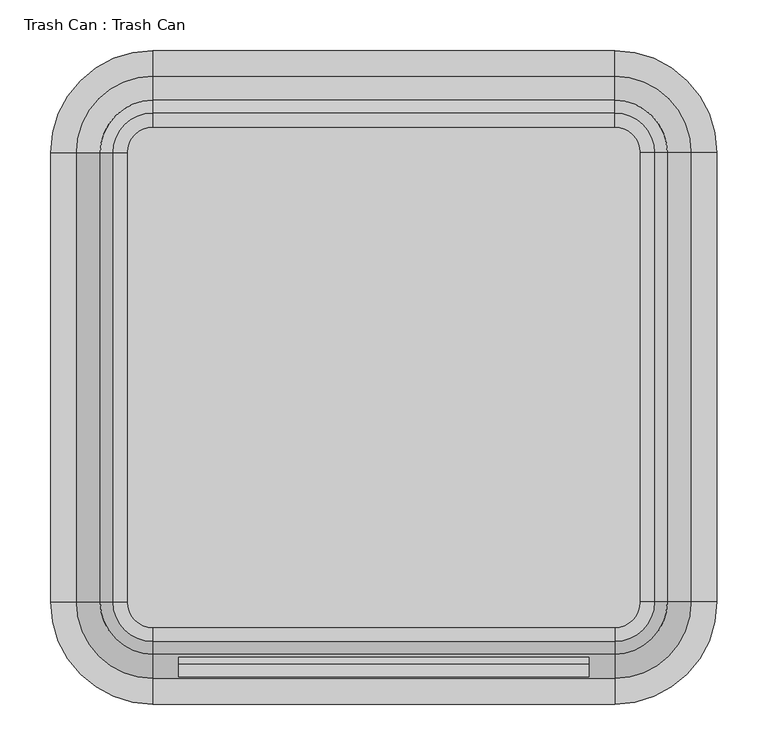
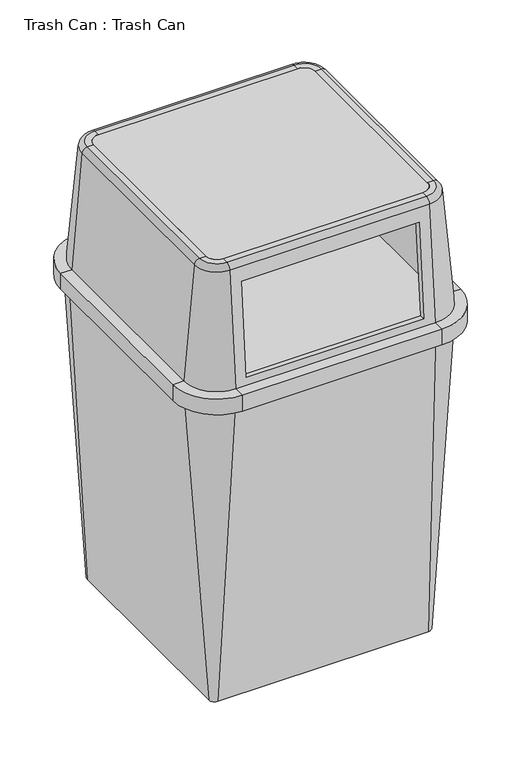
"""IFC4 building model written with IfcOpenShell, lengths in millimetres: geographic element geometry, Trash Can : Trash Can."""

from ifc_helpers import new_model, si_unit, point, frame, frame_2d, origin, place, context, project, spatial, polyline, circle_curve, ellipse_curve, trimmed, segment, composite_curve, outline, extrude, source, transform, mapped, element, save
from ifc_brep_helpers import plane_surface, cylinder_surface, revolved_surface, spline_surface, advanced_brep


def trash_can_trash_can_952d1acd(model_context):
    return source(origin(), model_context, "Body", "SolidModel", [
        advanced_brep(
        [(-254.0, 215.9, 1066.8), (-228.6, 241.3, 1066.8), (-228.6, 255.0625941, 1066.8), (-267.7625941, 215.9, 1066.8), (-254.0, 215.9, 1054.1), (-228.6, 241.3, 1054.1), (-267.7625941, 215.9, 1054.1), (-228.6, 255.0625941, 1054.1), (-292.6673476, 215.9, 769.437365), (-228.6, 279.9673476, 769.437365), (-317.0047535, 215.9, 769.437365), (-228.6, 304.3047535, 769.437365), (-317.0047535, 215.9, 744.037365), (-228.6, 304.3047535, 744.037365), (-329.7047535, 215.9, 744.037365), (-228.6, 317.0047535, 744.037365), (-329.7047535, 215.9, 782.137365), (-228.6, 317.0047535, 782.137365), (-304.3047535, 215.9, 782.137365), (-228.6, 291.6047535, 782.137365), (-280.4142668, 215.9, 1055.2068779), (-228.6, 267.7142668, 1055.2068779), (-267.7625941, -228.6, 1066.8), (-254.0, -228.6, 1066.8), (-254.0, -228.6, 1054.1), (-267.7625941, -228.6, 1054.1), (-292.6673476, -228.6, 769.437365), (-317.0047535, -228.6, 769.437365), (-317.0047535, -228.6, 744.037365), (-329.7047535, -228.6, 744.037365), (-329.7047535, -228.6, 782.137365), (-304.3047535, -228.6, 782.137365), (-280.4142668, -228.6, 1055.2068779), (-228.6, -267.7625941, 1066.8), (-228.6, -254.0, 1066.8), (-228.6, -254.0, 1054.1), (-228.6, -267.7625941, 1054.1), (-228.6, -292.6673476, 769.437365), (-228.6, -317.0047535, 769.437365), (-228.6, -317.0047535, 744.037365), (-228.6, -329.7047535, 744.037365), (-228.6, -329.7047535, 782.137365), (-228.6, -304.3047535, 782.137365), (-228.6, -280.4142668, 1055.2068779), (228.6, -267.7625941, 1066.8), (228.6, -254.0, 1066.8), (228.6, -254.0, 1054.1), (228.6, -267.7625941, 1054.1), (228.6, -292.6673476, 769.437365), (203.2, -290.0863084, 798.9387774), (203.2, -270.7170435, 1020.3304889), (-203.2, -270.7170435, 1020.3304889), (-203.2, -290.0863084, 798.9387774), (228.6, -317.0047535, 769.437365), (228.6, -317.0047535, 744.037365), (228.6, -329.7047535, 744.037365), (228.6, -329.7047535, 782.137365), (228.6, -304.3047535, 782.137365), (228.6, -280.4142668, 1055.2068779), (203.2, -283.3687161, 1021.4373669), (203.2, -302.7379811, 800.0456554), (-203.2, -302.7379811, 800.0456554), (-203.2, -283.3687161, 1021.4373669), (267.7625941, -228.6, 1066.8), (254.0, -228.6, 1066.8), (254.0, -228.6, 1054.1), (267.7625941, -228.6, 1054.1), (292.6673476, -228.6, 769.437365), (317.0047535, -228.6, 769.437365), (317.0047535, -228.6, 744.037365), (329.7047535, -228.6, 744.037365), (329.7047535, -228.6, 782.137365), (304.3047535, -228.6, 782.137365), (280.4142668, -228.6, 1055.2068779), (267.7625941, 215.9, 1066.8), (254.0, 215.9, 1066.8), (254.0, 215.9, 1054.1), (267.7625941, 215.9, 1054.1), (292.6673476, 215.9, 769.437365), (317.0047535, 215.9, 769.437365), (317.0047535, 215.9, 744.037365), (329.7047535, 215.9, 744.037365), (329.7047535, 215.9, 782.137365), (304.3047535, 215.9, 782.137365), (280.4142668, 215.9, 1055.2068779), (228.6, 255.0625941, 1066.8), (228.6, 241.3, 1066.8), (228.6, 241.3, 1054.1), (228.6, 255.0625941, 1054.1), (228.6, 279.9673476, 769.437365), (228.6, 304.3047535, 769.437365), (228.6, 304.3047535, 744.037365), (228.6, 317.0047535, 744.037365), (228.6, 317.0047535, 782.137365), (228.6, 291.6047535, 782.137365), (228.6, 267.7142668, 1055.2068779)],
        [
            (0, 1, circle_curve(frame((-228.6, 215.9, 1066.8), z_axis=(0.0, 0.0, -1.0), x_axis=(0.0, 1.0, 0.0)), 25.4)),
            (1, 2),
            (2, 3, circle_curve(frame((-228.6, 215.9, 1066.8), z_axis=(0.0, 0.0, 1.0), x_axis=(0.0, 1.0, 0.0)), 39.1625941)),
            (3, 0),
            (0, 4),
            (4, 5, circle_curve(frame((-228.6, 215.9, 1054.1), z_axis=(0.0, 0.0, -1.0), x_axis=(0.0, 1.0, 0.0)), 25.4)),
            (5, 1),
            (4, 6),
            (6, 7, circle_curve(frame((-228.6, 215.9, 1054.1), z_axis=(0.0, 0.0, -1.0), x_axis=(0.0, 1.0, 0.0)), 39.1625941)),
            (7, 5),
            (6, 8),
            (8, 9, circle_curve(frame((-228.6, 215.9, 769.437365), z_axis=(0.0, 0.0, -1.0), x_axis=(0.0, 1.0, 0.0)), 64.0673476)),
            (9, 7),
            (8, 10),
            (10, 11, circle_curve(frame((-228.6, 215.9, 769.437365), z_axis=(0.0, 0.0, -1.0), x_axis=(0.0, 1.0, 0.0)), 88.4047535)),
            (11, 9),
            (10, 12),
            (12, 13, circle_curve(frame((-228.6, 215.9, 744.037365), z_axis=(0.0, 0.0, -1.0), x_axis=(0.0, 1.0, 0.0)), 88.4047535)),
            (13, 11),
            (12, 14),
            (14, 15, circle_curve(frame((-228.6, 215.9, 744.037365), z_axis=(0.0, 0.0, -1.0), x_axis=(0.0, 1.0, 0.0)), 101.1047535)),
            (15, 13),
            (14, 16),
            (16, 17, circle_curve(frame((-228.6, 215.9, 782.137365), z_axis=(0.0, 0.0, -1.0), x_axis=(0.0, 1.0, 0.0)), 101.1047535)),
            (17, 15),
            (16, 18),
            (18, 19, circle_curve(frame((-228.6, 215.9, 782.137365), z_axis=(0.0, 0.0, -1.0), x_axis=(0.0, 1.0, 0.0)), 75.7047535)),
            (19, 17),
            (18, 20),
            (20, 21, circle_curve(frame((-228.6, 215.9, 1055.2068779), z_axis=(0.0, 0.0, -1.0), x_axis=(0.0, 1.0, 0.0)), 51.8142668)),
            (21, 19),
            (2, 21, circle_curve(frame((-228.6, 255.0625941, 1054.1), z_axis=(-1.0, 0.0, 0.0), x_axis=(0.0, -1.0, 0.0)), 12.7)),
            (20, 3, circle_curve(frame((-267.7625941, 215.9, 1054.1), z_axis=(0.0, 1.0, 0.0), x_axis=(1.0, 0.0, 0.0)), 12.7)),
            (3, 22),
            (22, 23),
            (23, 0),
            (23, 24),
            (24, 4),
            (24, 25),
            (25, 6),
            (25, 26),
            (26, 8),
            (26, 27),
            (27, 10),
            (27, 28),
            (28, 12),
            (28, 29),
            (29, 14),
            (29, 30),
            (30, 16),
            (30, 31),
            (31, 18),
            (31, 32),
            (32, 20),
            (32, 22, circle_curve(frame((-267.7625941, -228.6, 1054.1), z_axis=(0.0, 1.0, 0.0), x_axis=(1.0, 0.0, 0.0)), 12.7)),
            (22, 33, circle_curve(frame((-228.6, -228.6, 1066.8), z_axis=(0.0, 0.0, 1.0), x_axis=(-1.0, 0.0, 0.0)), 39.1625941)),
            (33, 34),
            (34, 23, circle_curve(frame((-228.6, -228.6, 1066.8), z_axis=(0.0, 0.0, -1.0), x_axis=(-1.0, 0.0, 0.0)), 25.4)),
            (34, 35),
            (35, 24, circle_curve(frame((-228.6, -228.6, 1054.1), z_axis=(0.0, 0.0, -1.0), x_axis=(-1.0, 0.0, 0.0)), 25.4)),
            (35, 36),
            (36, 25, circle_curve(frame((-228.6, -228.6, 1054.1), z_axis=(0.0, 0.0, -1.0), x_axis=(-1.0, 0.0, 0.0)), 39.1625941)),
            (36, 37),
            (37, 26, circle_curve(frame((-228.6, -228.6, 769.437365), z_axis=(0.0, 0.0, -1.0), x_axis=(-1.0, 0.0, 0.0)), 64.0673476)),
            (37, 38),
            (38, 27, circle_curve(frame((-228.6, -228.6, 769.437365), z_axis=(0.0, 0.0, -1.0), x_axis=(-1.0, 0.0, 0.0)), 88.4047535)),
            (38, 39),
            (39, 28, circle_curve(frame((-228.6, -228.6, 744.037365), z_axis=(0.0, 0.0, -1.0), x_axis=(-1.0, 0.0, 0.0)), 88.4047535)),
            (39, 40),
            (40, 29, circle_curve(frame((-228.6, -228.6, 744.037365), z_axis=(0.0, 0.0, -1.0), x_axis=(-1.0, 0.0, 0.0)), 101.1047535)),
            (40, 41),
            (41, 30, circle_curve(frame((-228.6, -228.6, 782.137365), z_axis=(0.0, 0.0, -1.0), x_axis=(-1.0, 0.0, 0.0)), 101.1047535)),
            (41, 42),
            (42, 31, circle_curve(frame((-228.6, -228.6, 782.137365), z_axis=(0.0, 0.0, -1.0), x_axis=(-1.0, 0.0, 0.0)), 75.7047535)),
            (42, 43),
            (43, 32, circle_curve(frame((-228.6, -228.6, 1055.2068779), z_axis=(0.0, 0.0, -1.0), x_axis=(-1.0, 0.0, 0.0)), 51.8142668)),
            (43, 33, circle_curve(frame((-228.6, -267.7625941, 1054.1), z_axis=(-1.0, 0.0, 0.0), x_axis=(0.0, 1.0, 0.0)), 12.7)),
            (33, 44),
            (44, 45),
            (45, 34),
            (45, 46),
            (46, 35),
            (46, 47),
            (47, 36),
            (47, 48),
            (48, 37),
            (49, 50),
            (50, 51),
            (51, 52),
            (52, 49),
            (48, 53),
            (53, 38),
            (53, 54),
            (54, 39),
            (54, 55),
            (55, 40),
            (55, 56),
            (56, 41),
            (56, 57),
            (57, 42),
            (57, 58),
            (58, 43),
            (59, 60),
            (60, 61),
            (61, 62),
            (62, 59),
            (58, 44, circle_curve(frame((228.6, -267.7625941, 1054.1), z_axis=(-1.0, 0.0, 0.0), x_axis=(0.0, 1.0, 0.0)), 12.7)),
            (44, 63, circle_curve(frame((228.6, -228.6, 1066.8), z_axis=(0.0, 0.0, 1.0), x_axis=(0.0, -1.0, 0.0)), 39.1625941)),
            (63, 64),
            (64, 45, circle_curve(frame((228.6, -228.6, 1066.8), z_axis=(0.0, 0.0, -1.0), x_axis=(0.0, -1.0, 0.0)), 25.4)),
            (64, 65),
            (65, 46, circle_curve(frame((228.6, -228.6, 1054.1), z_axis=(0.0, 0.0, -1.0), x_axis=(0.0, -1.0, 0.0)), 25.4)),
            (65, 66),
            (66, 47, circle_curve(frame((228.6, -228.6, 1054.1), z_axis=(0.0, 0.0, -1.0), x_axis=(0.0, -1.0, 0.0)), 39.1625941)),
            (66, 67),
            (67, 48, circle_curve(frame((228.6, -228.6, 769.437365), z_axis=(0.0, 0.0, -1.0), x_axis=(0.0, -1.0, 0.0)), 64.0673476)),
            (67, 68),
            (68, 53, circle_curve(frame((228.6, -228.6, 769.437365), z_axis=(0.0, 0.0, -1.0), x_axis=(0.0, -1.0, 0.0)), 88.4047535)),
            (68, 69),
            (69, 54, circle_curve(frame((228.6, -228.6, 744.037365), z_axis=(0.0, 0.0, -1.0), x_axis=(0.0, -1.0, 0.0)), 88.4047535)),
            (69, 70),
            (70, 55, circle_curve(frame((228.6, -228.6, 744.037365), z_axis=(0.0, 0.0, -1.0), x_axis=(0.0, -1.0, 0.0)), 101.1047535)),
            (70, 71),
            (71, 56, circle_curve(frame((228.6, -228.6, 782.137365), z_axis=(0.0, 0.0, -1.0), x_axis=(0.0, -1.0, 0.0)), 101.1047535)),
            (71, 72),
            (72, 57, circle_curve(frame((228.6, -228.6, 782.137365), z_axis=(0.0, 0.0, -1.0), x_axis=(0.0, -1.0, 0.0)), 75.7047535)),
            (72, 73),
            (73, 58, circle_curve(frame((228.6, -228.6, 1055.2068779), z_axis=(0.0, 0.0, -1.0), x_axis=(0.0, -1.0, 0.0)), 51.8142668)),
            (73, 63, circle_curve(frame((267.7625941, -228.6, 1054.1), z_axis=(0.0, -1.0, 0.0), x_axis=(-1.0, 0.0, 0.0)), 12.7)),
            (63, 74),
            (74, 75),
            (75, 64),
            (75, 76),
            (76, 65),
            (76, 77),
            (77, 66),
            (77, 78),
            (78, 67),
            (78, 79),
            (79, 68),
            (79, 80),
            (80, 69),
            (80, 81),
            (81, 70),
            (81, 82),
            (82, 71),
            (82, 83),
            (83, 72),
            (83, 84),
            (84, 73),
            (84, 74, circle_curve(frame((267.7625941, 215.9, 1054.1), z_axis=(0.0, -1.0, 0.0), x_axis=(-1.0, 0.0, 0.0)), 12.7)),
            (74, 85, circle_curve(frame((228.6, 215.9, 1066.8), z_axis=(0.0, 0.0, 1.0), x_axis=(1.0, 0.0, 0.0)), 39.1625941)),
            (85, 86),
            (86, 75, circle_curve(frame((228.6, 215.9, 1066.8), z_axis=(0.0, 0.0, -1.0), x_axis=(1.0, 0.0, 0.0)), 25.4)),
            (86, 87),
            (87, 76, circle_curve(frame((228.6, 215.9, 1054.1), z_axis=(0.0, 0.0, -1.0), x_axis=(1.0, 0.0, 0.0)), 25.4)),
            (87, 88),
            (88, 77, circle_curve(frame((228.6, 215.9, 1054.1), z_axis=(0.0, 0.0, -1.0), x_axis=(1.0, 0.0, 0.0)), 39.1625941)),
            (88, 89),
            (89, 78, circle_curve(frame((228.6, 215.9, 769.437365), z_axis=(0.0, 0.0, -1.0), x_axis=(1.0, 0.0, 0.0)), 64.0673476)),
            (89, 90),
            (90, 79, circle_curve(frame((228.6, 215.9, 769.437365), z_axis=(0.0, 0.0, -1.0), x_axis=(1.0, 0.0, 0.0)), 88.4047535)),
            (90, 91),
            (91, 80, circle_curve(frame((228.6, 215.9, 744.037365), z_axis=(0.0, 0.0, -1.0), x_axis=(1.0, 0.0, 0.0)), 88.4047535)),
            (91, 92),
            (92, 81, circle_curve(frame((228.6, 215.9, 744.037365), z_axis=(0.0, 0.0, -1.0), x_axis=(1.0, 0.0, 0.0)), 101.1047535)),
            (92, 93),
            (93, 82, circle_curve(frame((228.6, 215.9, 782.137365), z_axis=(0.0, 0.0, -1.0), x_axis=(1.0, 0.0, 0.0)), 101.1047535)),
            (93, 94),
            (94, 83, circle_curve(frame((228.6, 215.9, 782.137365), z_axis=(0.0, 0.0, -1.0), x_axis=(1.0, 0.0, 0.0)), 75.7047535)),
            (94, 95),
            (95, 84, circle_curve(frame((228.6, 215.9, 1055.2068779), z_axis=(0.0, 0.0, -1.0), x_axis=(1.0, 0.0, 0.0)), 51.8142668)),
            (95, 85, circle_curve(frame((228.6, 255.0625941, 1054.1), z_axis=(1.0, 0.0, 0.0), x_axis=(0.0, -1.0, 0.0)), 12.7)),
            (1, 86),
            (85, 2),
            (5, 87),
            (7, 88),
            (9, 89),
            (11, 90),
            (13, 91),
            (15, 92),
            (17, 93),
            (19, 94),
            (21, 95),
            (59, 50),
            (49, 60),
            (52, 61),
            (51, 62),
        ],
        [
            plane_surface(frame((-228.6, 215.9, 1066.8), z_axis=(0.0, 0.0, 1.0), x_axis=(0.0, 1.0, 0.0))),
            revolved_surface(polyline([(-228.6, 241.3, 1066.8), (-228.6, 241.3, 1054.1)]), (-228.6, 215.9, 0.0), (0.0, 0.0, 1.0)),
            plane_surface(frame((-228.6, 215.9, 1054.1), z_axis=(0.0, 0.0, -1.0), x_axis=(0.0, 1.0, 0.0))),
            revolved_surface(polyline([(-228.6, 255.0625941, 1054.1), (-228.6, 279.9673476, 769.437365)]), (-228.6, 215.9, 0.0), (0.0, 0.0, 1.0)),
            plane_surface(frame((-228.6, 215.9, 769.437365), z_axis=(0.0, 0.0, -1.0), x_axis=(0.0, 1.0, 0.0))),
            revolved_surface(polyline([(-228.6, 304.3047535, 769.437365), (-228.6, 304.3047535, 744.037365)]), (-228.6, 215.9, 0.0), (0.0, 0.0, 1.0)),
            plane_surface(frame((-228.6, 215.9, 744.037365), z_axis=(0.0, 0.0, -1.0), x_axis=(0.0, 1.0, 0.0))),
            cylinder_surface(frame((-228.6, 215.9, 0.0), z_axis=(0.0, 0.0, 1.0), x_axis=(0.0, 1.0, 0.0)), 101.1047535),
            plane_surface(frame((-228.6, 215.9, 782.137365), z_axis=(0.0, 0.0, 1.0), x_axis=(0.0, 1.0, 0.0))),
            revolved_surface(polyline([(-228.6, 291.6047535, 782.137365), (-228.6, 267.7142668, 1055.2068779)]), (-228.6, 215.9, 0.0), (0.0, 0.0, 1.0)),
            revolved_surface(trimmed(ellipse_curve(frame((-228.6, 255.0625941, 1054.1), z_axis=(1.0, 0.0, 0.0), x_axis=(0.0, -1.0, 0.0)), 12.7, 12.7), [point((-228.6, 267.7142668, 1055.2068779))], [point((-228.6, 255.0625941, 1066.8))], True, "CARTESIAN"), (-228.6, 215.9, 0.0), (0.0, 0.0, 1.0)),
            plane_surface(frame((-267.7625941, 215.9, 1066.8), z_axis=(0.0, 0.0, 1.0), x_axis=(0.0, -1.0, 0.0))),
            plane_surface(frame((-254.0, 215.9, 1066.8), z_axis=(1.0, 0.0, 0.0), x_axis=(0.0, -1.0, 0.0))),
            plane_surface(frame((-254.0, 215.9, 1054.1), z_axis=(0.0, 0.0, -1.0), x_axis=(0.0, -1.0, 0.0))),
            plane_surface(frame((-267.7625941, 215.9, 1054.1), z_axis=(0.9961946980917451, 0.0, -0.08715574274766279), x_axis=(0.0, -1.0, 0.0))),
            plane_surface(frame((-292.6673476, 215.9, 769.437365), z_axis=(0.0, 0.0, -1.0), x_axis=(0.0, -1.0, 0.0))),
            plane_surface(frame((-317.0047535, 215.9, 769.437365), z_axis=(1.0, 0.0, 0.0), x_axis=(0.0, -1.0, 0.0))),
            plane_surface(frame((-317.0047535, 215.9, 744.037365), z_axis=(0.0, 0.0, -1.0), x_axis=(0.0, -1.0, 0.0))),
            plane_surface(frame((-329.7047535, 215.9, 744.037365), z_axis=(-1.0, 0.0, 0.0), x_axis=(0.0, -1.0, 0.0))),
            plane_surface(frame((-329.7047535, 215.9, 782.137365), z_axis=(0.0, 0.0, 1.0), x_axis=(0.0, -1.0, 0.0))),
            plane_surface(frame((-304.3047535, 215.9, 782.137365), z_axis=(-0.9961946980917452, 0.0, 0.08715574274766147), x_axis=(0.0, -1.0, 0.0))),
            cylinder_surface(frame((-267.7625941, 215.9, 1054.1), z_axis=(0.0, 1.0, 0.0), x_axis=(1.0, 0.0, 0.0)), 12.7),
            plane_surface(frame((-228.6, -228.6, 1066.8), z_axis=(0.0, 0.0, 1.0), x_axis=(-1.0, 0.0, 0.0))),
            revolved_surface(polyline([(-254.0, -228.6, 1066.8), (-254.0, -228.6, 1054.1)]), (-228.6, -228.6, 0.0), (0.0, 0.0, 1.0)),
            plane_surface(frame((-228.6, -228.6, 1054.1), z_axis=(0.0, 0.0, -1.0), x_axis=(-1.0, 0.0, 0.0))),
            revolved_surface(polyline([(-267.7625941, -228.6, 1054.1), (-292.6673476, -228.6, 769.437365)]), (-228.6, -228.6, 0.0), (0.0, 0.0, 1.0)),
            plane_surface(frame((-228.6, -228.6, 769.437365), z_axis=(0.0, 0.0, -1.0), x_axis=(-1.0, 0.0, 0.0))),
            revolved_surface(polyline([(-317.0047535, -228.6, 769.437365), (-317.0047535, -228.6, 744.037365)]), (-228.6, -228.6, 0.0), (0.0, 0.0, 1.0)),
            plane_surface(frame((-228.6, -228.6, 744.037365), z_axis=(0.0, 0.0, -1.0), x_axis=(-1.0, 0.0, 0.0))),
            cylinder_surface(frame((-228.6, -228.6, 0.0), z_axis=(0.0, 0.0, 1.0), x_axis=(-1.0, 0.0, 0.0)), 101.1047535),
            plane_surface(frame((-228.6, -228.6, 782.137365), z_axis=(0.0, 0.0, 1.0), x_axis=(-1.0, 0.0, 0.0))),
            revolved_surface(polyline([(-304.3047535, -228.6, 782.137365), (-280.4142668, -228.6, 1055.2068779)]), (-228.6, -228.6, 0.0), (0.0, 0.0, 1.0)),
            revolved_surface(trimmed(ellipse_curve(frame((-267.7625941, -228.6, 1054.1), z_axis=(0.0, 1.0, 0.0), x_axis=(1.0, 0.0, 0.0)), 12.7, 12.7), [point((-280.4142668, -228.6, 1055.2068779))], [point((-267.7625941, -228.6, 1066.8))], True, "CARTESIAN"), (-228.6, -228.6, 0.0), (0.0, 0.0, 1.0)),
            plane_surface(frame((-228.6, -267.7625941, 1066.8), z_axis=(0.0, 0.0, 1.0), x_axis=(1.0, 0.0, 0.0))),
            plane_surface(frame((-228.6, -254.0, 1066.8), z_axis=(0.0, 1.0, 0.0), x_axis=(1.0, 0.0, 0.0))),
            plane_surface(frame((-228.6, -254.0, 1054.1), z_axis=(0.0, 0.0, -1.0), x_axis=(1.0, 0.0, 0.0))),
            plane_surface(frame((-228.6, -267.7625941, 1054.1), z_axis=(0.0, 0.9961946980917451, -0.08715574274766279), x_axis=(1.0, 0.0, 0.0))),
            plane_surface(frame((-228.6, -292.6673476, 769.437365), z_axis=(0.0, 0.0, -1.0), x_axis=(1.0, 0.0, 0.0))),
            plane_surface(frame((-228.6, -317.0047535, 769.437365), z_axis=(0.0, 1.0, 0.0), x_axis=(1.0, 0.0, 0.0))),
            plane_surface(frame((-228.6, -317.0047535, 744.037365), z_axis=(0.0, 0.0, -1.0), x_axis=(1.0, 0.0, 0.0))),
            plane_surface(frame((-228.6, -329.7047535, 744.037365), z_axis=(0.0, -1.0, 0.0), x_axis=(1.0, 0.0, 0.0))),
            plane_surface(frame((-228.6, -329.7047535, 782.137365), z_axis=(0.0, 0.0, 1.0), x_axis=(1.0, 0.0, 0.0))),
            plane_surface(frame((-228.6, -304.3047535, 782.137365), z_axis=(0.0, -0.9961946980917452, 0.08715574274766147), x_axis=(1.0, 0.0, 0.0))),
            cylinder_surface(frame((-228.6, -267.7625941, 1054.1), z_axis=(-1.0, 0.0, 0.0), x_axis=(0.0, 1.0, 0.0)), 12.7),
            plane_surface(frame((228.6, -228.6, 1066.8), z_axis=(0.0, 0.0, 1.0), x_axis=(0.0, -1.0, 0.0))),
            revolved_surface(polyline([(228.6, -254.0, 1066.8), (228.6, -254.0, 1054.1)]), (228.6, -228.6, 0.0), (0.0, 0.0, 1.0)),
            plane_surface(frame((228.6, -228.6, 1054.1), z_axis=(0.0, 0.0, -1.0), x_axis=(0.0, -1.0, 0.0))),
            revolved_surface(polyline([(228.6, -267.7625941, 1054.1), (228.6, -292.6673476, 769.437365)]), (228.6, -228.6, 0.0), (0.0, 0.0, 1.0)),
            plane_surface(frame((228.6, -228.6, 769.437365), z_axis=(0.0, 0.0, -1.0), x_axis=(0.0, -1.0, 0.0))),
            revolved_surface(polyline([(228.6, -317.0047535, 769.437365), (228.6, -317.0047535, 744.037365)]), (228.6, -228.6, 0.0), (0.0, 0.0, 1.0)),
            plane_surface(frame((228.6, -228.6, 744.037365), z_axis=(0.0, 0.0, -1.0), x_axis=(0.0, -1.0, 0.0))),
            cylinder_surface(frame((228.6, -228.6, 0.0), z_axis=(0.0, 0.0, 1.0), x_axis=(0.0, -1.0, 0.0)), 101.1047535),
            plane_surface(frame((228.6, -228.6, 782.137365), z_axis=(0.0, 0.0, 1.0), x_axis=(0.0, -1.0, 0.0))),
            revolved_surface(polyline([(228.6, -304.3047535, 782.137365), (228.6, -280.4142668, 1055.2068779)]), (228.6, -228.6, 0.0), (0.0, 0.0, 1.0)),
            revolved_surface(trimmed(ellipse_curve(frame((228.6, -267.7625941, 1054.1), z_axis=(-1.0, 0.0, 0.0), x_axis=(0.0, 1.0, 0.0)), 12.7, 12.7), [point((228.6, -280.4142668, 1055.2068779))], [point((228.6, -267.7625941, 1066.8))], True, "CARTESIAN"), (228.6, -228.6, 0.0), (0.0, 0.0, 1.0)),
            plane_surface(frame((267.7625941, -228.6, 1066.8), z_axis=(0.0, 0.0, 1.0), x_axis=(0.0, 1.0, 0.0))),
            plane_surface(frame((254.0, -228.6, 1066.8), z_axis=(-1.0, 0.0, 0.0), x_axis=(0.0, 1.0, 0.0))),
            plane_surface(frame((254.0, -228.6, 1054.1), z_axis=(0.0, 0.0, -1.0), x_axis=(0.0, 1.0, 0.0))),
            plane_surface(frame((267.7625941, -228.6, 1054.1), z_axis=(-0.9961946980917451, 0.0, -0.08715574274766279), x_axis=(0.0, 1.0, 0.0))),
            plane_surface(frame((292.6673476, -228.6, 769.437365), z_axis=(0.0, 0.0, -1.0), x_axis=(0.0, 1.0, 0.0))),
            plane_surface(frame((317.0047535, -228.6, 769.437365), z_axis=(-1.0, 0.0, 0.0), x_axis=(0.0, 1.0, 0.0))),
            plane_surface(frame((317.0047535, -228.6, 744.037365), z_axis=(0.0, 0.0, -1.0), x_axis=(0.0, 1.0, 0.0))),
            plane_surface(frame((329.7047535, -228.6, 744.037365), z_axis=(1.0, 0.0, 0.0), x_axis=(0.0, 1.0, 0.0))),
            plane_surface(frame((329.7047535, -228.6, 782.137365), z_axis=(0.0, 0.0, 1.0), x_axis=(0.0, 1.0, 0.0))),
            plane_surface(frame((304.3047535, -228.6, 782.137365), z_axis=(0.9961946980917452, 0.0, 0.08715574274766147), x_axis=(0.0, 1.0, 0.0))),
            cylinder_surface(frame((267.7625941, -228.6, 1054.1), z_axis=(0.0, -1.0, 0.0), x_axis=(-1.0, 0.0, 0.0)), 12.7),
            plane_surface(frame((228.6, 215.9, 1066.8), z_axis=(0.0, 0.0, 1.0), x_axis=(1.0, 0.0, 0.0))),
            revolved_surface(polyline([(254.0, 215.9, 1066.8), (254.0, 215.9, 1054.1)]), (228.6, 215.9, 0.0), (0.0, 0.0, 1.0)),
            plane_surface(frame((228.6, 215.9, 1054.1), z_axis=(0.0, 0.0, -1.0), x_axis=(1.0, 0.0, 0.0))),
            revolved_surface(polyline([(267.7625941, 215.9, 1054.1), (292.6673476, 215.9, 769.437365)]), (228.6, 215.9, 0.0), (0.0, 0.0, 1.0)),
            plane_surface(frame((228.6, 215.9, 769.437365), z_axis=(0.0, 0.0, -1.0), x_axis=(1.0, 0.0, 0.0))),
            revolved_surface(polyline([(317.0047535, 215.9, 769.437365), (317.0047535, 215.9, 744.037365)]), (228.6, 215.9, 0.0), (0.0, 0.0, 1.0)),
            plane_surface(frame((228.6, 215.9, 744.037365), z_axis=(0.0, 0.0, -1.0), x_axis=(1.0, 0.0, 0.0))),
            cylinder_surface(frame((228.6, 215.9, 0.0), z_axis=(0.0, 0.0, 1.0), x_axis=(1.0, 0.0, 0.0)), 101.1047535),
            plane_surface(frame((228.6, 215.9, 782.137365), z_axis=(0.0, 0.0, 1.0), x_axis=(1.0, 0.0, 0.0))),
            revolved_surface(polyline([(304.3047535, 215.9, 782.137365), (280.4142668, 215.9, 1055.2068779)]), (228.6, 215.9, 0.0), (0.0, 0.0, 1.0)),
            revolved_surface(trimmed(ellipse_curve(frame((267.7625941, 215.9, 1054.1), z_axis=(0.0, -1.0, 0.0), x_axis=(-1.0, 0.0, 0.0)), 12.7, 12.7), [point((280.4142668, 215.9, 1055.2068779))], [point((267.7625941, 215.9, 1066.8))], True, "CARTESIAN"), (228.6, 215.9, 0.0), (0.0, 0.0, 1.0)),
            plane_surface(frame((228.6, 255.0625941, 1066.8), z_axis=(0.0, 0.0, 1.0), x_axis=(-1.0, 0.0, 0.0))),
            plane_surface(frame((228.6, 241.3, 1066.8), z_axis=(0.0, -1.0, 0.0), x_axis=(-1.0, 0.0, 0.0))),
            plane_surface(frame((228.6, 241.3, 1054.1), z_axis=(0.0, 0.0, -1.0), x_axis=(-1.0, 0.0, 0.0))),
            plane_surface(frame((228.6, 255.0625941, 1054.1), z_axis=(0.0, -0.9961946980917451, -0.08715574274766279), x_axis=(-1.0, 0.0, 0.0))),
            plane_surface(frame((228.6, 279.9673476, 769.437365), z_axis=(0.0, 0.0, -1.0), x_axis=(-1.0, 0.0, 0.0))),
            plane_surface(frame((228.6, 304.3047535, 769.437365), z_axis=(0.0, -1.0, 0.0), x_axis=(-1.0, 0.0, 0.0))),
            plane_surface(frame((228.6, 304.3047535, 744.037365), z_axis=(0.0, 0.0, -1.0), x_axis=(-1.0, 0.0, 0.0))),
            plane_surface(frame((228.6, 317.0047535, 744.037365), z_axis=(0.0, 1.0, 0.0), x_axis=(-1.0, 0.0, 0.0))),
            plane_surface(frame((228.6, 317.0047535, 782.137365), z_axis=(0.0, 0.0, 1.0), x_axis=(-1.0, 0.0, 0.0))),
            plane_surface(frame((228.6, 291.6047535, 782.137365), z_axis=(0.0, 0.9961946980917452, 0.08715574274766147), x_axis=(-1.0, 0.0, 0.0))),
            cylinder_surface(frame((228.6, 255.0625941, 1054.1), z_axis=(1.0, 0.0, 0.0), x_axis=(0.0, -1.0, 0.0)), 12.7),
            plane_surface(frame((203.2, -213.4252032, 1015.3181024), z_axis=(-1.0, 0.0, 0.0), x_axis=(0.0, -0.9961946980917452, 0.08715574274766175))),
            plane_surface(frame((203.2, -232.7944681, 793.9263909), z_axis=(0.0, 0.08715574274766175, 0.9961946980917452), x_axis=(0.0, -0.9961946980917452, 0.08715574274766175))),
            plane_surface(frame((-203.2, -232.7944681, 793.9263909), z_axis=(1.0, 0.0, 0.0), x_axis=(0.0, -0.9961946980917452, 0.08715574274766175))),
            plane_surface(frame((-203.2, -213.4252032, 1015.3181024), z_axis=(0.0, -0.08715574274766175, -0.9961946980917452), x_axis=(0.0, -0.9961946980917452, 0.08715574274766175))),
        ],
        [
            (0, [[1, 2, 3, 4]]),
            (1, [[-1, 5, 6, 7]]),
            (2, [[-6, 8, 9, 10]]),
            (3, [[-9, 11, 12, 13]]),
            (4, [[-12, 14, 15, 16]]),
            (5, [[-15, 17, 18, 19]]),
            (6, [[-18, 20, 21, 22]]),
            (7, [[-21, 23, 24, 25]]),
            (8, [[-24, 26, 27, 28]]),
            (9, [[-27, 29, 30, 31]]),
            (10, [[-3, 32, -30, 33]]),
            (11, [[-4, 34, 35, 36]]),
            (12, [[-5, -36, 37, 38]]),
            (13, [[-8, -38, 39, 40]]),
            (14, [[-11, -40, 41, 42]]),
            (15, [[-14, -42, 43, 44]]),
            (16, [[-17, -44, 45, 46]]),
            (17, [[-20, -46, 47, 48]]),
            (18, [[-23, -48, 49, 50]]),
            (19, [[-26, -50, 51, 52]]),
            (20, [[-29, -52, 53, 54]]),
            (21, [[-33, -54, 55, -34]]),
            (22, [[-35, 56, 57, 58]]),
            (23, [[-37, -58, 59, 60]]),
            (24, [[-39, -60, 61, 62]]),
            (25, [[-41, -62, 63, 64]]),
            (26, [[-43, -64, 65, 66]]),
            (27, [[-45, -66, 67, 68]]),
            (28, [[-47, -68, 69, 70]]),
            (29, [[-49, -70, 71, 72]]),
            (30, [[-51, -72, 73, 74]]),
            (31, [[-53, -74, 75, 76]]),
            (32, [[-55, -76, 77, -56]]),
            (33, [[-57, 78, 79, 80]]),
            (34, [[-59, -80, 81, 82]]),
            (35, [[-61, -82, 83, 84]]),
            (36, [[-63, -84, 85, 86], [87, 88, 89, 90]]),
            (37, [[-65, -86, 91, 92]]),
            (38, [[-67, -92, 93, 94]]),
            (39, [[-69, -94, 95, 96]]),
            (40, [[-71, -96, 97, 98]]),
            (41, [[-73, -98, 99, 100]]),
            (42, [[-75, -100, 101, 102], [103, 104, 105, 106]]),
            (43, [[-77, -102, 107, -78]]),
            (44, [[-79, 108, 109, 110]]),
            (45, [[-81, -110, 111, 112]]),
            (46, [[-83, -112, 113, 114]]),
            (47, [[-85, -114, 115, 116]]),
            (48, [[-91, -116, 117, 118]]),
            (49, [[-93, -118, 119, 120]]),
            (50, [[-95, -120, 121, 122]]),
            (51, [[-97, -122, 123, 124]]),
            (52, [[-99, -124, 125, 126]]),
            (53, [[-101, -126, 127, 128]]),
            (54, [[-107, -128, 129, -108]]),
            (55, [[-109, 130, 131, 132]]),
            (56, [[-111, -132, 133, 134]]),
            (57, [[-113, -134, 135, 136]]),
            (58, [[-115, -136, 137, 138]]),
            (59, [[-117, -138, 139, 140]]),
            (60, [[-119, -140, 141, 142]]),
            (61, [[-121, -142, 143, 144]]),
            (62, [[-123, -144, 145, 146]]),
            (63, [[-125, -146, 147, 148]]),
            (64, [[-127, -148, 149, 150]]),
            (65, [[-129, -150, 151, -130]]),
            (66, [[-131, 152, 153, 154]]),
            (67, [[-133, -154, 155, 156]]),
            (68, [[-135, -156, 157, 158]]),
            (69, [[-137, -158, 159, 160]]),
            (70, [[-139, -160, 161, 162]]),
            (71, [[-141, -162, 163, 164]]),
            (72, [[-143, -164, 165, 166]]),
            (73, [[-145, -166, 167, 168]]),
            (74, [[-147, -168, 169, 170]]),
            (75, [[-149, -170, 171, 172]]),
            (76, [[-151, -172, 173, -152]]),
            (77, [[-2, 174, -153, 175]]),
            (78, [[-7, 176, -155, -174]]),
            (79, [[-10, 177, -157, -176]]),
            (80, [[-13, 178, -159, -177]]),
            (81, [[-16, 179, -161, -178]]),
            (82, [[-19, 180, -163, -179]]),
            (83, [[-22, 181, -165, -180]]),
            (84, [[-25, 182, -167, -181]]),
            (85, [[-28, 183, -169, -182]]),
            (86, [[-31, 184, -171, -183]]),
            (87, [[-32, -175, -173, -184]]),
            (88, [[185, -87, 186, -103]]),
            (89, [[-186, -90, 187, -104]]),
            (90, [[-187, -89, 188, -105]]),
            (91, [[-185, -106, -188, -88]]),
        ],
    ),
        extrude(outline(composite_curve([segment(trimmed(circle_curve(frame_2d((241.3, 228.6)), 12.7), [point((241.3, 241.3))], [point((254.0, 228.6))], False, "CARTESIAN"), True, "CONTINUOUS"), segment(polyline([(254.0, 228.6), (254.0, -228.6)]), True, "CONTINUOUS"), segment(trimmed(circle_curve(frame_2d((228.6, -228.6)), 25.4), [point((254.0, -228.6))], [point((228.6, -254.0))], False, "CARTESIAN"), True, "CONTINUOUS"), segment(polyline([(228.6, -254.0), (-228.6, -254.0)]), True, "CONTINUOUS"), segment(trimmed(circle_curve(frame_2d((-228.6, -228.6)), 25.4), [point((-228.6, -254.0))], [point((-254.0, -228.6))], False, "CARTESIAN"), True, "CONTINUOUS"), segment(polyline([(-254.0, -228.6), (-254.0, 215.9)]), True, "CONTINUOUS"), segment(trimmed(circle_curve(frame_2d((-228.6, 215.9)), 25.4), [point((-254.0, 215.9))], [point((-228.6, 241.3))], False, "CARTESIAN"), True, "CONTINUOUS"), segment(polyline([(-228.6, 241.3), (241.3, 241.3)]), True, "CONTINUOUS")], self_intersect=False)), frame((0.0, 0.0, 1054.1), z_axis=(0.0, 0.0, 1.0), x_axis=(1.0, 0.0, 0.0)), (0.0, 0.0, 1.0), 12.7),
        advanced_brep(
        [(228.6, 304.8, 762.0), (-228.6, 304.8, 762.0), (-304.8, 228.6, 762.0), (-304.8, -228.6, 762.0), (-228.6, -304.8, 762.0), (228.6, -304.8, 762.0), (304.8, -228.6, 762.0), (304.8, 228.6, 762.0), (241.3, 254.0, 0.0), (254.0, 241.3, 0.0), (254.0, -241.3, 0.0), (241.3, -254.0, 0.0), (-241.3, -254.0, 0.0), (-254.0, -241.3, 0.0), (-254.0, 241.3, 0.0), (-241.3, 254.0, 0.0)],
        [
            (0, 1),
            (1, 2, circle_curve(frame((-228.6, 228.6, 762.0), z_axis=(0.0, 0.0, 1.0), x_axis=(1.0, 0.0, 0.0)), 76.2)),
            (2, 3),
            (3, 4, circle_curve(frame((-228.6, -228.6, 762.0), z_axis=(0.0, 0.0, 1.0), x_axis=(1.0, 0.0, 0.0)), 76.2)),
            (4, 5),
            (5, 6, circle_curve(frame((228.6, -228.6, 762.0), z_axis=(0.0, 0.0, 1.0), x_axis=(1.0, 0.0, 0.0)), 76.2)),
            (6, 7),
            (7, 0, circle_curve(frame((228.6, 228.6, 762.0), z_axis=(0.0, 0.0, 1.0), x_axis=(1.0, 0.0, 0.0)), 76.2)),
            (8, 9, circle_curve(frame((241.3, 241.3, 0.0), z_axis=(0.0, 0.0, -1.0), x_axis=(1.0, 0.0, 0.0)), 12.7)),
            (9, 10),
            (10, 11, circle_curve(frame((241.3, -241.3, 0.0), z_axis=(0.0, 0.0, -1.0), x_axis=(1.0, 0.0, 0.0)), 12.7)),
            (11, 12),
            (12, 13, circle_curve(frame((-241.3, -241.3, 0.0), z_axis=(0.0, 0.0, -1.0), x_axis=(1.0, 0.0, 0.0)), 12.7)),
            (13, 14),
            (14, 15, circle_curve(frame((-241.3, 241.3, 0.0), z_axis=(0.0, 0.0, -1.0), x_axis=(1.0, 0.0, 0.0)), 12.7)),
            (15, 8),
            (15, 1),
            (0, 8),
            (14, 2),
            (13, 3),
            (12, 4),
            (11, 5),
            (10, 6),
            (9, 7),
        ],
        [
            plane_surface(frame((0.0, 0.0, 762.0), z_axis=(0.0, 0.0, 1.0), x_axis=(-1.0, 0.0, 0.0))),
            plane_surface(frame((0.0, 0.0, 0.0), z_axis=(0.0, 0.0, -1.0), x_axis=(-1.0, 0.0, 0.0))),
            plane_surface(frame((0.0, 254.0, 0.0), z_axis=(0.0, 0.9977851578566089, -0.0665190105237736), x_axis=(-1.0, 0.0, 0.0))),
            spline_surface(2, 1, [[(-241.3, 254.0, 0.0), (-228.6, 304.8, 762.0)], [(-254.0, 254.0, 0.0), (-304.8, 304.8, 762.0)], [(-254.0, 241.3, 0.0), (-304.8, 228.6, 762.0)]], [3, 3], [2, 2], [0.0, 1.0], [0.0, 1.0], weights=[[1.0, 1.0], [0.7071067811865476, 0.7071067811865476], [1.0, 1.0]]),
            plane_surface(frame((-254.0, 0.0, 0.0), z_axis=(-0.9977851578566089, 0.0, -0.06651901052377489), x_axis=(0.0, -1.0, 0.0))),
            spline_surface(2, 1, [[(-254.0, -241.3, 0.0), (-304.8, -228.6, 762.0)], [(-254.0, -254.0, 0.0), (-304.8, -304.8, 762.0)], [(-241.3, -254.0, 0.0), (-228.6, -304.8, 762.0)]], [3, 3], [2, 2], [0.0, 1.0], [0.0, 1.0], weights=[[1.0, 1.0], [0.7071067811865476, 0.7071067811865476], [1.0, 1.0]]),
            plane_surface(frame((0.0, -254.0, 0.0), z_axis=(0.0, -0.9977851578566089, -0.06651901052377414), x_axis=(1.0, 0.0, 0.0))),
            spline_surface(2, 1, [[(241.3, -254.0, 0.0), (228.6, -304.8, 762.0)], [(254.0, -254.0, 0.0), (304.8, -304.8, 762.0)], [(254.0, -241.3, 0.0), (304.8, -228.6, 762.0)]], [3, 3], [2, 2], [0.0, 1.0], [0.0, 1.0], weights=[[1.0, 1.0], [0.7071067811865476, 0.7071067811865476], [1.0, 1.0]]),
            plane_surface(frame((254.0, 0.0, 0.0), z_axis=(0.9977851578566089, 0.0, -0.0665190105237748), x_axis=(0.0, 1.0, 0.0))),
            spline_surface(2, 1, [[(254.0, 241.3, 0.0), (304.8, 228.6, 762.0)], [(254.0, 254.0, 0.0), (304.8, 304.8, 762.0)], [(241.3, 254.0, 0.0), (228.6, 304.8, 762.0)]], [3, 3], [2, 2], [0.0, 1.0], [0.0, 1.0], weights=[[1.0, 1.0], [0.7071067811865476, 0.7071067811865476], [1.0, 1.0]]),
        ],
        [
            (0, [[1, 2, 3, 4, 5, 6, 7, 8]]),
            (1, [[9, 10, 11, 12, 13, 14, 15, 16]]),
            (2, [[-16, 17, -1, 18]]),
            (3, [[-15, 19, -2, -17]]),
            (4, [[-14, 20, -3, -19]]),
            (5, [[-13, 21, -4, -20]]),
            (6, [[-12, 22, -5, -21]]),
            (7, [[-11, 23, -6, -22]]),
            (8, [[-10, 24, -7, -23]]),
            (9, [[-9, -18, -8, -24]]),
        ],
    ),
    ])


if __name__ == "__main__":
    model = new_model("IFC4")
    model_context = context("Model", 3, world=origin())
    ifc_project = project(units=[si_unit("LENGTHUNIT", "METRE", prefix="MILLI")], contexts=[model_context])
    site = spatial("IfcSite", under=ifc_project)
    building = spatial("IfcBuilding", under=site)
    placement = place(None, origin())
    trash_can_trash_can_shape = trash_can_trash_can_952d1acd(model_context)
    element("IfcGeographicElement", 1, ObjectType="Trash Can : Trash Can", at=placement, inside=building, context=model_context, shape_type="MappedRepresentation", body=[
        mapped(trash_can_trash_can_shape, transform((0.0, 0.0, 0.0), x_axis=(1.0, 0.0, 0.0), y_axis=(0.0, 1.0, 0.0), z_axis=(0.0, 0.0, 1.0))),
    ])
    save(model, "model.ifc")

# Revit data of these elements
# Type "Trash Can : Trash Can"
#   Assembly Code = "G2040900"
# Element 1 (IfcGeographicElement, "Trash Can : Trash Can")
#   Materials on its faces: "Plastic - Gray, Dark", "Plastic, Opaque Black"
# Materials
#   "Plastic - Gray, Dark": class "Plastic", colour RGB 134 134 134, transparency 0
#   "Plastic, Opaque Black": class "Plastic", colour RGB 0 0 0, transparency 0.05, Description = "Plastic, generic, opaque black", Cost = 0
